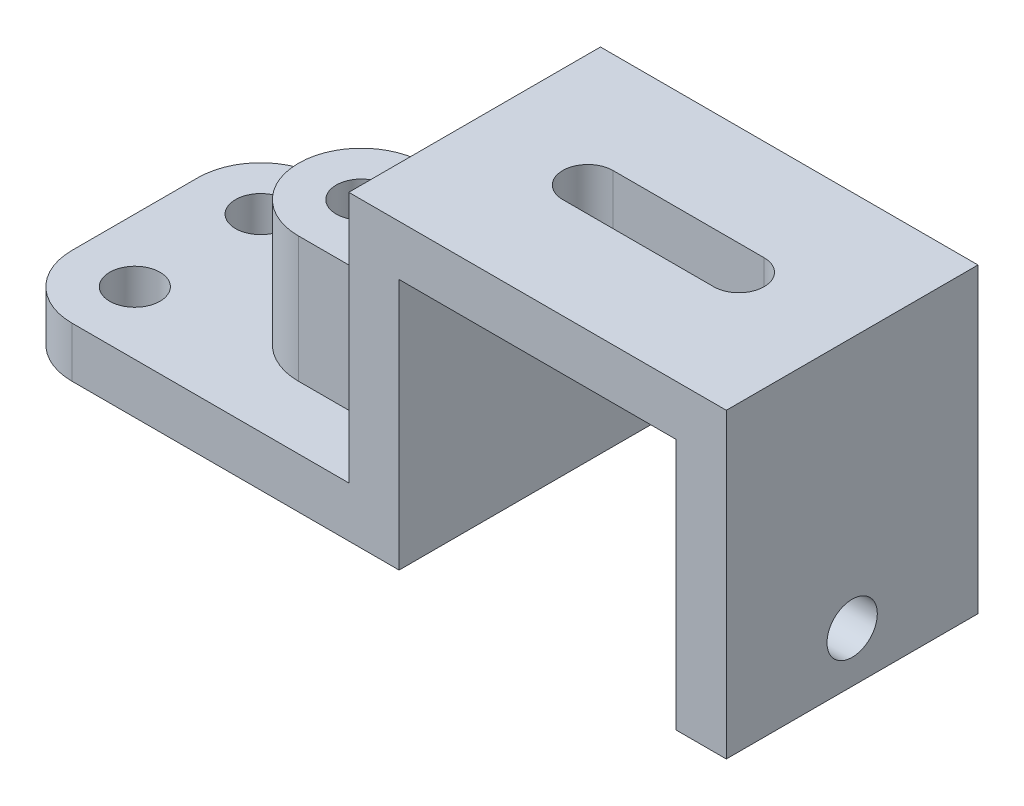
ISO-10303-21;
HEADER;
FILE_DESCRIPTION(('STEP AP214'),'2;1');
FILE_NAME('part.step','',(''),(''),'','','');
FILE_SCHEMA(('AUTOMOTIVE_DESIGN { 1 0 10303 214 1 1 1 1 }'));
ENDSEC;
DATA;
#1=APPLICATION_CONTEXT('core data for automotive mechanical design processes');
#2=APPLICATION_PROTOCOL_DEFINITION('international standard','automotive_design',2000,#1);
#3=PRODUCT_CONTEXT('',#1,'mechanical');
#4=PRODUCT('Part','Part','',(#3));
#5=PRODUCT_RELATED_PRODUCT_CATEGORY('part','',(#4));
#6=PRODUCT_DEFINITION_FORMATION('','',#4);
#7=PRODUCT_DEFINITION_CONTEXT('part definition',#1,'design');
#8=PRODUCT_DEFINITION('design','',#6,#7);
#9=PRODUCT_DEFINITION_SHAPE('','',#8);
#10=(LENGTH_UNIT() NAMED_UNIT(*) SI_UNIT(.MILLI.,.METRE.));
#11=(NAMED_UNIT(*) PLANE_ANGLE_UNIT() SI_UNIT($,.RADIAN.));
#12=(NAMED_UNIT(*) SI_UNIT($,.STERADIAN.) SOLID_ANGLE_UNIT());
#13=UNCERTAINTY_MEASURE_WITH_UNIT(LENGTH_MEASURE(1.E-05),#10,'distance_accuracy_value','');
#14=(GEOMETRIC_REPRESENTATION_CONTEXT(3) GLOBAL_UNCERTAINTY_ASSIGNED_CONTEXT((#13)) GLOBAL_UNIT_ASSIGNED_CONTEXT((#10,
#11,#12)) REPRESENTATION_CONTEXT('',''));
#15=CARTESIAN_POINT('',(0.,0.,0.));
#16=DIRECTION('',(0.,0.,1.));
#17=DIRECTION('',(1.,0.,0.));
#18=AXIS2_PLACEMENT_3D('',#15,#16,#17);
#19=CARTESIAN_POINT('',(121.5,17.9999999999999,45.));
#20=DIRECTION('',(1.,0.,0.));
#21=DIRECTION('',(0.,0.,-1.));
#22=AXIS2_PLACEMENT_3D('',#19,#20,#21);
#23=PLANE('',#22);
#24=DIRECTION('',(0.,-1.,0.));
#25=VECTOR('',#24,1.);
#26=CARTESIAN_POINT('',(121.5,62.9999999999999,22.5));
#27=LINE('',#26,#25);
#28=CARTESIAN_POINT('',(121.5,62.9999999999999,22.5));
#29=VERTEX_POINT('',#28);
#30=CARTESIAN_POINT('',(121.5,17.9999999999999,22.5));
#31=VERTEX_POINT('',#30);
#32=EDGE_CURVE('E187',#29,#31,#27,.T.);
#33=ORIENTED_EDGE('',*,*,#32,.T.);
#34=DIRECTION('',(0.,0.,-1.));
#35=VECTOR('',#34,1.);
#36=CARTESIAN_POINT('',(121.5,17.9999999999999,45.));
#37=LINE('',#36,#35);
#38=CARTESIAN_POINT('',(121.5,17.9999999999999,45.));
#39=VERTEX_POINT('',#38);
#40=EDGE_CURVE('E276',#39,#31,#37,.T.);
#41=ORIENTED_EDGE('',*,*,#40,.F.);
#42=DIRECTION('',(0.,-1.,0.));
#43=VECTOR('',#42,1.);
#44=CARTESIAN_POINT('',(121.5,17.9999999999999,45.));
#45=LINE('',#44,#43);
#46=CARTESIAN_POINT('',(121.5,108.,45.));
#47=VERTEX_POINT('',#46);
#48=EDGE_CURVE('E253',#47,#39,#45,.T.);
#49=ORIENTED_EDGE('',*,*,#48,.F.);
#50=DIRECTION('',(0.,0.,-1.));
#51=VECTOR('',#50,1.);
#52=CARTESIAN_POINT('',(121.5,108.,45.));
#53=LINE('',#52,#51);
#54=CARTESIAN_POINT('',(121.5,108.,-45.));
#55=VERTEX_POINT('',#54);
#56=EDGE_CURVE('E285',#47,#55,#53,.T.);
#57=ORIENTED_EDGE('',*,*,#56,.T.);
#58=DIRECTION('',(0.,-1.,0.));
#59=VECTOR('',#58,1.);
#60=CARTESIAN_POINT('',(121.5,17.9999999999999,-45.));
#61=LINE('',#60,#59);
#62=CARTESIAN_POINT('',(121.5,17.9999999999999,-45.));
#63=VERTEX_POINT('',#62);
#64=EDGE_CURVE('E267',#55,#63,#61,.T.);
#65=ORIENTED_EDGE('',*,*,#64,.T.);
#66=CARTESIAN_POINT('',(121.5,17.9999999999999,-22.4999999999999));
#67=VERTEX_POINT('',#66);
#68=EDGE_CURVE('E279',#67,#63,#37,.T.);
#69=ORIENTED_EDGE('',*,*,#68,.F.);
#70=DIRECTION('',(0.,-1.,0.));
#71=VECTOR('',#70,1.);
#72=CARTESIAN_POINT('',(121.5,62.9999999999999,-22.5));
#73=LINE('',#72,#71);
#74=CARTESIAN_POINT('',(121.5,62.9999999999999,-22.5));
#75=VERTEX_POINT('',#74);
#76=EDGE_CURVE('E211',#75,#67,#73,.T.);
#77=ORIENTED_EDGE('',*,*,#76,.F.);
#78=DIRECTION('',(0.,0.,-1.));
#79=VECTOR('',#78,1.);
#80=CARTESIAN_POINT('',(121.5,62.9999999999999,-22.5));
#81=LINE('',#80,#79);
#82=EDGE_CURVE('E191',#29,#75,#81,.T.);
#83=ORIENTED_EDGE('',*,*,#82,.F.);
#84=EDGE_LOOP('',(#33,#41,#49,#57,#65,#69,#77,#83));
#85=FACE_BOUND('',#84,.T.);
#86=ADVANCED_FACE('F39',(#85),#23,.F.);
#87=CARTESIAN_POINT('',(0.,17.9999999999999,45.));
#88=DIRECTION('',(0.,-1.,0.));
#89=DIRECTION('',(0.,0.,-1.));
#90=AXIS2_PLACEMENT_3D('',#87,#88,#89);
#91=PLANE('',#90);
#92=CARTESIAN_POINT('',(22.5,17.9999999999999,-22.5));
#93=DIRECTION('',(0.,1.,0.));
#94=DIRECTION('',(0.,0.,1.));
#95=AXIS2_PLACEMENT_3D('',#92,#93,#94);
#96=CIRCLE('',#95,9.);
#97=CARTESIAN_POINT('',(22.5,17.9999999999999,-13.5));
#98=VERTEX_POINT('',#97);
#99=EDGE_CURVE('E327',#98,#98,#96,.T.);
#100=ORIENTED_EDGE('',*,*,#99,.F.);
#101=EDGE_LOOP('',(#100));
#102=FACE_BOUND('',#101,.T.);
#103=CARTESIAN_POINT('',(22.5,17.9999999999999,22.5));
#104=DIRECTION('',(0.,1.,0.));
#105=DIRECTION('',(0.,0.,1.));
#106=AXIS2_PLACEMENT_3D('',#103,#104,#105);
#107=CIRCLE('',#106,9.);
#108=CARTESIAN_POINT('',(22.5,17.9999999999999,31.5));
#109=VERTEX_POINT('',#108);
#110=EDGE_CURVE('E331',#109,#109,#107,.T.);
#111=ORIENTED_EDGE('',*,*,#110,.F.);
#112=EDGE_LOOP('',(#111));
#113=FACE_BOUND('',#112,.T.);
#114=DIRECTION('',(-1.,0.,0.));
#115=VECTOR('',#114,1.);
#116=CARTESIAN_POINT('',(0.,17.9999999999999,-45.));
#117=LINE('',#116,#115);
#118=CARTESIAN_POINT('',(22.5,17.9999999999999,-45.));
#119=VERTEX_POINT('',#118);
#120=EDGE_CURVE('E239',#63,#119,#117,.T.);
#121=ORIENTED_EDGE('',*,*,#120,.T.);
#122=CARTESIAN_POINT('',(22.5,17.9999999999999,-22.5));
#123=DIRECTION('',(0.,-1.,0.));
#124=DIRECTION('',(0.,0.,-1.));
#125=AXIS2_PLACEMENT_3D('',#122,#123,#124);
#126=CIRCLE('',#125,22.5);
#127=CARTESIAN_POINT('',(0.,17.9999999999999,-22.5));
#128=VERTEX_POINT('',#127);
#129=EDGE_CURVE('E48',#119,#128,#126,.F.);
#130=ORIENTED_EDGE('',*,*,#129,.T.);
#131=DIRECTION('',(0.,0.,-1.));
#132=VECTOR('',#131,1.);
#133=CARTESIAN_POINT('',(0.,17.9999999999999,45.));
#134=LINE('',#133,#132);
#135=CARTESIAN_POINT('',(0.,17.9999999999999,22.5));
#136=VERTEX_POINT('',#135);
#137=EDGE_CURVE('E274',#136,#128,#134,.T.);
#138=ORIENTED_EDGE('',*,*,#137,.F.);
#139=CARTESIAN_POINT('',(22.5,17.9999999999999,22.5));
#140=DIRECTION('',(0.,-1.,0.));
#141=DIRECTION('',(0.,0.,-1.));
#142=AXIS2_PLACEMENT_3D('',#139,#140,#141);
#143=CIRCLE('',#142,22.5);
#144=CARTESIAN_POINT('',(22.5,17.9999999999999,45.));
#145=VERTEX_POINT('',#144);
#146=EDGE_CURVE('E57',#136,#145,#143,.F.);
#147=ORIENTED_EDGE('',*,*,#146,.T.);
#148=DIRECTION('',(-1.,0.,0.));
#149=VECTOR('',#148,1.);
#150=CARTESIAN_POINT('',(0.,17.9999999999999,45.));
#151=LINE('',#150,#149);
#152=EDGE_CURVE('E251',#39,#145,#151,.T.);
#153=ORIENTED_EDGE('',*,*,#152,.F.);
#154=ORIENTED_EDGE('',*,*,#40,.T.);
#155=DIRECTION('',(1.,0.,0.));
#156=VECTOR('',#155,1.);
#157=CARTESIAN_POINT('',(81.,17.9999999999999,22.5));
#158=LINE('',#157,#156);
#159=CARTESIAN_POINT('',(81.,17.9999999999999,22.5));
#160=VERTEX_POINT('',#159);
#161=EDGE_CURVE('E351',#160,#31,#158,.T.);
#162=ORIENTED_EDGE('',*,*,#161,.F.);
#163=CARTESIAN_POINT('',(81.,17.9999999999999,0.));
#164=DIRECTION('',(0.,1.,0.));
#165=DIRECTION('',(0.,0.,1.));
#166=AXIS2_PLACEMENT_3D('',#163,#164,#165);
#167=CIRCLE('',#166,22.5);
#168=CARTESIAN_POINT('',(81.,17.9999999999999,-22.5));
#169=VERTEX_POINT('',#168);
#170=EDGE_CURVE('E206',#169,#160,#167,.T.);
#171=ORIENTED_EDGE('',*,*,#170,.F.);
#172=DIRECTION('',(-1.,0.,0.));
#173=VECTOR('',#172,1.);
#174=CARTESIAN_POINT('',(81.,17.9999999999999,-22.5));
#175=LINE('',#174,#173);
#176=EDGE_CURVE('E201',#67,#169,#175,.T.);
#177=ORIENTED_EDGE('',*,*,#176,.F.);
#178=ORIENTED_EDGE('',*,*,#68,.T.);
#179=EDGE_LOOP('',(#121,#130,#138,#147,#153,#154,#162,#171,#177,#178));
#180=FACE_BOUND('',#179,.T.);
#181=ADVANCED_FACE('F361',(#102,#113,#180),#91,.F.);
#182=CARTESIAN_POINT('',(139.5,0.,45.));
#183=DIRECTION('',(0.,1.,0.));
#184=DIRECTION('',(-1.,0.,0.));
#185=AXIS2_PLACEMENT_3D('',#182,#183,#184);
#186=PLANE('',#185);
#187=CARTESIAN_POINT('',(22.5,0.,-22.5));
#188=DIRECTION('',(0.,1.,0.));
#189=DIRECTION('',(-1.,0.,0.));
#190=AXIS2_PLACEMENT_3D('',#187,#188,#189);
#191=CIRCLE('',#190,9.);
#192=CARTESIAN_POINT('',(13.5,0.,-22.5));
#193=VERTEX_POINT('',#192);
#194=EDGE_CURVE('E43',#193,#193,#191,.T.);
#195=ORIENTED_EDGE('',*,*,#194,.T.);
#196=EDGE_LOOP('',(#195));
#197=FACE_BOUND('',#196,.T.);
#198=CARTESIAN_POINT('',(22.5,0.,22.5));
#199=DIRECTION('',(0.,1.,0.));
#200=DIRECTION('',(-1.,0.,0.));
#201=AXIS2_PLACEMENT_3D('',#198,#199,#200);
#202=CIRCLE('',#201,9.);
#203=CARTESIAN_POINT('',(13.5,0.,22.5));
#204=VERTEX_POINT('',#203);
#205=EDGE_CURVE('E326',#204,#204,#202,.T.);
#206=ORIENTED_EDGE('',*,*,#205,.T.);
#207=EDGE_LOOP('',(#206));
#208=FACE_BOUND('',#207,.T.);
#209=CARTESIAN_POINT('',(81.,0.,0.));
#210=DIRECTION('',(0.,1.,0.));
#211=DIRECTION('',(-1.,0.,0.));
#212=AXIS2_PLACEMENT_3D('',#209,#210,#211);
#213=CIRCLE('',#212,9.);
#214=CARTESIAN_POINT('',(72.,0.,0.));
#215=VERTEX_POINT('',#214);
#216=EDGE_CURVE('E347',#215,#215,#213,.T.);
#217=ORIENTED_EDGE('',*,*,#216,.T.);
#218=EDGE_LOOP('',(#217));
#219=FACE_BOUND('',#218,.T.);
#220=DIRECTION('',(0.,0.,-1.));
#221=VECTOR('',#220,1.);
#222=CARTESIAN_POINT('',(0.,0.,45.));
#223=LINE('',#222,#221);
#224=CARTESIAN_POINT('',(0.,0.,22.5));
#225=VERTEX_POINT('',#224);
#226=CARTESIAN_POINT('',(0.,0.,-22.5));
#227=VERTEX_POINT('',#226);
#228=EDGE_CURVE('E254',#225,#227,#223,.T.);
#229=ORIENTED_EDGE('',*,*,#228,.T.);
#230=CARTESIAN_POINT('',(22.5,0.,-22.5));
#231=DIRECTION('',(0.,1.,0.));
#232=DIRECTION('',(-1.,0.,0.));
#233=AXIS2_PLACEMENT_3D('',#230,#231,#232);
#234=CIRCLE('',#233,22.5);
#235=CARTESIAN_POINT('',(22.5,0.,-45.));
#236=VERTEX_POINT('',#235);
#237=EDGE_CURVE('E325',#227,#236,#234,.F.);
#238=ORIENTED_EDGE('',*,*,#237,.T.);
#239=DIRECTION('',(1.,0.,0.));
#240=VECTOR('',#239,1.);
#241=CARTESIAN_POINT('',(139.5,0.,-45.));
#242=LINE('',#241,#240);
#243=CARTESIAN_POINT('',(139.5,0.,-45.));
#244=VERTEX_POINT('',#243);
#245=EDGE_CURVE('E232',#236,#244,#242,.T.);
#246=ORIENTED_EDGE('',*,*,#245,.T.);
#247=DIRECTION('',(0.,0.,-1.));
#248=VECTOR('',#247,1.);
#249=CARTESIAN_POINT('',(139.5,0.,45.));
#250=LINE('',#249,#248);
#251=CARTESIAN_POINT('',(139.5,0.,45.));
#252=VERTEX_POINT('',#251);
#253=EDGE_CURVE('E297',#252,#244,#250,.T.);
#254=ORIENTED_EDGE('',*,*,#253,.F.);
#255=DIRECTION('',(1.,0.,0.));
#256=VECTOR('',#255,1.);
#257=CARTESIAN_POINT('',(139.5,0.,45.));
#258=LINE('',#257,#256);
#259=CARTESIAN_POINT('',(22.5,0.,45.));
#260=VERTEX_POINT('',#259);
#261=EDGE_CURVE('E237',#260,#252,#258,.T.);
#262=ORIENTED_EDGE('',*,*,#261,.F.);
#263=CARTESIAN_POINT('',(22.5,0.,22.5));
#264=DIRECTION('',(0.,1.,0.));
#265=DIRECTION('',(-1.,0.,0.));
#266=AXIS2_PLACEMENT_3D('',#263,#264,#265);
#267=CIRCLE('',#266,22.5);
#268=EDGE_CURVE('E319',#260,#225,#267,.F.);
#269=ORIENTED_EDGE('',*,*,#268,.T.);
#270=EDGE_LOOP('',(#229,#238,#246,#254,#262,#269));
#271=FACE_BOUND('',#270,.T.);
#272=ADVANCED_FACE('F404',(#197,#208,#219,#271),#186,.F.);
#273=CARTESIAN_POINT('',(139.5,89.9999999999999,45.));
#274=DIRECTION('',(-1.,0.,0.));
#275=DIRECTION('',(0.,0.,1.));
#276=AXIS2_PLACEMENT_3D('',#273,#274,#275);
#277=PLANE('',#276);
#278=DIRECTION('',(0.,1.,0.));
#279=VECTOR('',#278,1.);
#280=CARTESIAN_POINT('',(139.5,89.9999999999999,-45.));
#281=LINE('',#280,#279);
#282=CARTESIAN_POINT('',(139.5,89.9999999999999,-45.));
#283=VERTEX_POINT('',#282);
#284=EDGE_CURVE('E260',#244,#283,#281,.T.);
#285=ORIENTED_EDGE('',*,*,#284,.T.);
#286=DIRECTION('',(0.,0.,-1.));
#287=VECTOR('',#286,1.);
#288=CARTESIAN_POINT('',(139.5,89.9999999999999,45.));
#289=LINE('',#288,#287);
#290=CARTESIAN_POINT('',(139.5,89.9999999999999,45.));
#291=VERTEX_POINT('',#290);
#292=EDGE_CURVE('E300',#291,#283,#289,.T.);
#293=ORIENTED_EDGE('',*,*,#292,.F.);
#294=DIRECTION('',(0.,1.,0.));
#295=VECTOR('',#294,1.);
#296=CARTESIAN_POINT('',(139.5,89.9999999999999,45.));
#297=LINE('',#296,#295);
#298=EDGE_CURVE('E236',#252,#291,#297,.T.);
#299=ORIENTED_EDGE('',*,*,#298,.F.);
#300=ORIENTED_EDGE('',*,*,#253,.T.);
#301=EDGE_LOOP('',(#285,#293,#299,#300));
#302=FACE_BOUND('',#301,.T.);
#303=ADVANCED_FACE('F397',(#302),#277,.F.);
#304=CARTESIAN_POINT('',(238.5,89.9999999999999,45.));
#305=DIRECTION('',(0.,1.,0.));
#306=DIRECTION('',(-1.,0.,0.));
#307=AXIS2_PLACEMENT_3D('',#304,#305,#306);
#308=PLANE('',#307);
#309=DIRECTION('',(-1.,0.,0.));
#310=VECTOR('',#309,1.);
#311=CARTESIAN_POINT('',(238.5,89.9999999999999,-9.00000000000001));
#312=LINE('',#311,#310);
#313=CARTESIAN_POINT('',(216.,89.9999999999999,-9.00000000000001));
#314=VERTEX_POINT('',#313);
#315=CARTESIAN_POINT('',(162.,89.9999999999999,-9.));
#316=VERTEX_POINT('',#315);
#317=EDGE_CURVE('E229',#314,#316,#312,.T.);
#318=ORIENTED_EDGE('',*,*,#317,.T.);
#319=CARTESIAN_POINT('',(162.,89.9999999999999,0.));
#320=DIRECTION('',(0.,1.,0.));
#321=DIRECTION('',(-1.,0.,0.));
#322=AXIS2_PLACEMENT_3D('',#319,#320,#321);
#323=CIRCLE('',#322,9.);
#324=CARTESIAN_POINT('',(162.,89.9999999999999,9.));
#325=VERTEX_POINT('',#324);
#326=EDGE_CURVE('E235',#316,#325,#323,.T.);
#327=ORIENTED_EDGE('',*,*,#326,.T.);
#328=DIRECTION('',(1.,0.,0.));
#329=VECTOR('',#328,1.);
#330=CARTESIAN_POINT('',(238.5,89.9999999999999,9.));
#331=LINE('',#330,#329);
#332=CARTESIAN_POINT('',(216.,89.9999999999999,9.00000000000001));
#333=VERTEX_POINT('',#332);
#334=EDGE_CURVE('E217',#325,#333,#331,.T.);
#335=ORIENTED_EDGE('',*,*,#334,.T.);
#336=CARTESIAN_POINT('',(216.,89.9999999999999,0.));
#337=DIRECTION('',(0.,1.,0.));
#338=DIRECTION('',(-1.,0.,0.));
#339=AXIS2_PLACEMENT_3D('',#336,#337,#338);
#340=CIRCLE('',#339,9.);
#341=EDGE_CURVE('E228',#333,#314,#340,.T.);
#342=ORIENTED_EDGE('',*,*,#341,.T.);
#343=EDGE_LOOP('',(#318,#327,#335,#342));
#344=FACE_BOUND('',#343,.T.);
#345=DIRECTION('',(1.,0.,0.));
#346=VECTOR('',#345,1.);
#347=CARTESIAN_POINT('',(238.5,89.9999999999999,-45.));
#348=LINE('',#347,#346);
#349=CARTESIAN_POINT('',(238.5,89.9999999999999,-45.));
#350=VERTEX_POINT('',#349);
#351=EDGE_CURVE('E259',#283,#350,#348,.T.);
#352=ORIENTED_EDGE('',*,*,#351,.T.);
#353=DIRECTION('',(0.,0.,-1.));
#354=VECTOR('',#353,1.);
#355=CARTESIAN_POINT('',(238.5,89.9999999999999,45.));
#356=LINE('',#355,#354);
#357=CARTESIAN_POINT('',(238.5,89.9999999999999,45.));
#358=VERTEX_POINT('',#357);
#359=EDGE_CURVE('E294',#358,#350,#356,.T.);
#360=ORIENTED_EDGE('',*,*,#359,.F.);
#361=DIRECTION('',(1.,0.,0.));
#362=VECTOR('',#361,1.);
#363=CARTESIAN_POINT('',(238.5,89.9999999999999,45.));
#364=LINE('',#363,#362);
#365=EDGE_CURVE('E243',#291,#358,#364,.T.);
#366=ORIENTED_EDGE('',*,*,#365,.F.);
#367=ORIENTED_EDGE('',*,*,#292,.T.);
#368=EDGE_LOOP('',(#352,#360,#366,#367));
#369=FACE_BOUND('',#368,.T.);
#370=ADVANCED_FACE('F392',(#344,#369),#308,.F.);
#371=CARTESIAN_POINT('',(238.5,0.,45.));
#372=DIRECTION('',(1.,0.,0.));
#373=DIRECTION('',(0.,0.,-1.));
#374=AXIS2_PLACEMENT_3D('',#371,#372,#373);
#375=PLANE('',#374);
#376=CARTESIAN_POINT('',(238.5,18.,0.));
#377=DIRECTION('',(1.,0.,0.));
#378=DIRECTION('',(0.,0.,-1.));
#379=AXIS2_PLACEMENT_3D('',#376,#377,#378);
#380=CIRCLE('',#379,9.);
#381=CARTESIAN_POINT('',(238.5,18.,-9.));
#382=VERTEX_POINT('',#381);
#383=EDGE_CURVE('E339',#382,#382,#380,.T.);
#384=ORIENTED_EDGE('',*,*,#383,.T.);
#385=EDGE_LOOP('',(#384));
#386=FACE_BOUND('',#385,.T.);
#387=DIRECTION('',(0.,-1.,0.));
#388=VECTOR('',#387,1.);
#389=CARTESIAN_POINT('',(238.5,0.,-45.));
#390=LINE('',#389,#388);
#391=CARTESIAN_POINT('',(238.5,0.,-45.));
#392=VERTEX_POINT('',#391);
#393=EDGE_CURVE('E261',#350,#392,#390,.T.);
#394=ORIENTED_EDGE('',*,*,#393,.T.);
#395=DIRECTION('',(0.,0.,-1.));
#396=VECTOR('',#395,1.);
#397=CARTESIAN_POINT('',(238.5,0.,45.));
#398=LINE('',#397,#396);
#399=CARTESIAN_POINT('',(238.5,0.,45.));
#400=VERTEX_POINT('',#399);
#401=EDGE_CURVE('E292',#400,#392,#398,.T.);
#402=ORIENTED_EDGE('',*,*,#401,.F.);
#403=DIRECTION('',(0.,-1.,0.));
#404=VECTOR('',#403,1.);
#405=CARTESIAN_POINT('',(238.5,0.,45.));
#406=LINE('',#405,#404);
#407=EDGE_CURVE('E241',#358,#400,#406,.T.);
#408=ORIENTED_EDGE('',*,*,#407,.F.);
#409=ORIENTED_EDGE('',*,*,#359,.T.);
#410=EDGE_LOOP('',(#394,#402,#408,#409));
#411=FACE_BOUND('',#410,.T.);
#412=ADVANCED_FACE('F388',(#386,#411),#375,.F.);
#413=CARTESIAN_POINT('',(256.5,0.,45.));
#414=DIRECTION('',(0.,1.,0.));
#415=DIRECTION('',(0.,0.,1.));
#416=AXIS2_PLACEMENT_3D('',#413,#414,#415);
#417=PLANE('',#416);
#418=DIRECTION('',(1.,0.,0.));
#419=VECTOR('',#418,1.);
#420=CARTESIAN_POINT('',(256.5,0.,-45.));
#421=LINE('',#420,#419);
#422=CARTESIAN_POINT('',(256.5,0.,-45.));
#423=VERTEX_POINT('',#422);
#424=EDGE_CURVE('E263',#392,#423,#421,.T.);
#425=ORIENTED_EDGE('',*,*,#424,.T.);
#426=DIRECTION('',(0.,0.,-1.));
#427=VECTOR('',#426,1.);
#428=CARTESIAN_POINT('',(256.5,0.,45.));
#429=LINE('',#428,#427);
#430=CARTESIAN_POINT('',(256.5,0.,45.));
#431=VERTEX_POINT('',#430);
#432=EDGE_CURVE('E286',#431,#423,#429,.T.);
#433=ORIENTED_EDGE('',*,*,#432,.F.);
#434=DIRECTION('',(1.,0.,0.));
#435=VECTOR('',#434,1.);
#436=CARTESIAN_POINT('',(256.5,0.,45.));
#437=LINE('',#436,#435);
#438=EDGE_CURVE('E242',#400,#431,#437,.T.);
#439=ORIENTED_EDGE('',*,*,#438,.F.);
#440=ORIENTED_EDGE('',*,*,#401,.T.);
#441=EDGE_LOOP('',(#425,#433,#439,#440));
#442=FACE_BOUND('',#441,.T.);
#443=ADVANCED_FACE('F387',(#442),#417,.F.);
#444=CARTESIAN_POINT('',(256.5,108.,45.));
#445=DIRECTION('',(-1.,0.,0.));
#446=DIRECTION('',(0.,0.,1.));
#447=AXIS2_PLACEMENT_3D('',#444,#445,#446);
#448=PLANE('',#447);
#449=CARTESIAN_POINT('',(256.5,18.,0.));
#450=DIRECTION('',(1.,0.,0.));
#451=DIRECTION('',(0.,0.,-1.));
#452=AXIS2_PLACEMENT_3D('',#449,#450,#451);
#453=CIRCLE('',#452,9.);
#454=CARTESIAN_POINT('',(256.5,18.,-9.));
#455=VERTEX_POINT('',#454);
#456=EDGE_CURVE('E648',#455,#455,#453,.T.);
#457=ORIENTED_EDGE('',*,*,#456,.F.);
#458=EDGE_LOOP('',(#457));
#459=FACE_BOUND('',#458,.T.);
#460=DIRECTION('',(0.,1.,0.));
#461=VECTOR('',#460,1.);
#462=CARTESIAN_POINT('',(256.5,108.,-45.));
#463=LINE('',#462,#461);
#464=CARTESIAN_POINT('',(256.5,108.,-45.));
#465=VERTEX_POINT('',#464);
#466=EDGE_CURVE('E264',#423,#465,#463,.T.);
#467=ORIENTED_EDGE('',*,*,#466,.T.);
#468=DIRECTION('',(0.,0.,-1.));
#469=VECTOR('',#468,1.);
#470=CARTESIAN_POINT('',(256.5,108.,45.));
#471=LINE('',#470,#469);
#472=CARTESIAN_POINT('',(256.5,108.,45.));
#473=VERTEX_POINT('',#472);
#474=EDGE_CURVE('E282',#473,#465,#471,.T.);
#475=ORIENTED_EDGE('',*,*,#474,.F.);
#476=DIRECTION('',(0.,1.,0.));
#477=VECTOR('',#476,1.);
#478=CARTESIAN_POINT('',(256.5,108.,45.));
#479=LINE('',#478,#477);
#480=EDGE_CURVE('E250',#431,#473,#479,.T.);
#481=ORIENTED_EDGE('',*,*,#480,.F.);
#482=ORIENTED_EDGE('',*,*,#432,.T.);
#483=EDGE_LOOP('',(#467,#475,#481,#482));
#484=FACE_BOUND('',#483,.T.);
#485=ADVANCED_FACE('F385',(#459,#484),#448,.F.);
#486=CARTESIAN_POINT('',(121.5,108.,45.));
#487=DIRECTION('',(0.,-1.,0.));
#488=DIRECTION('',(0.,0.,-1.));
#489=AXIS2_PLACEMENT_3D('',#486,#487,#488);
#490=PLANE('',#489);
#491=DIRECTION('',(-1.,0.,0.));
#492=VECTOR('',#491,1.);
#493=CARTESIAN_POINT('',(121.5,108.,9.00000000000001));
#494=LINE('',#493,#492);
#495=CARTESIAN_POINT('',(216.,108.,9.));
#496=VERTEX_POINT('',#495);
#497=CARTESIAN_POINT('',(162.,108.,9.00000000000001));
#498=VERTEX_POINT('',#497);
#499=EDGE_CURVE('E301',#496,#498,#494,.T.);
#500=ORIENTED_EDGE('',*,*,#499,.T.);
#501=CARTESIAN_POINT('',(162.,108.,0.));
#502=DIRECTION('',(0.,-1.,0.));
#503=DIRECTION('',(0.,0.,-1.));
#504=AXIS2_PLACEMENT_3D('',#501,#502,#503);
#505=CIRCLE('',#504,9.);
#506=CARTESIAN_POINT('',(162.,108.,-9.));
#507=VERTEX_POINT('',#506);
#508=EDGE_CURVE('E315',#498,#507,#505,.T.);
#509=ORIENTED_EDGE('',*,*,#508,.T.);
#510=DIRECTION('',(1.,0.,0.));
#511=VECTOR('',#510,1.);
#512=CARTESIAN_POINT('',(121.5,108.,-8.99999999999999));
#513=LINE('',#512,#511);
#514=CARTESIAN_POINT('',(216.,108.,-9.00000000000001));
#515=VERTEX_POINT('',#514);
#516=EDGE_CURVE('E310',#507,#515,#513,.T.);
#517=ORIENTED_EDGE('',*,*,#516,.T.);
#518=CARTESIAN_POINT('',(216.,108.,0.));
#519=DIRECTION('',(0.,-1.,0.));
#520=DIRECTION('',(0.,0.,-1.));
#521=AXIS2_PLACEMENT_3D('',#518,#519,#520);
#522=CIRCLE('',#521,9.);
#523=EDGE_CURVE('E308',#515,#496,#522,.T.);
#524=ORIENTED_EDGE('',*,*,#523,.T.);
#525=EDGE_LOOP('',(#500,#509,#517,#524));
#526=FACE_BOUND('',#525,.T.);
#527=DIRECTION('',(-1.,0.,0.));
#528=VECTOR('',#527,1.);
#529=CARTESIAN_POINT('',(121.5,108.,-45.));
#530=LINE('',#529,#528);
#531=EDGE_CURVE('E270',#465,#55,#530,.T.);
#532=ORIENTED_EDGE('',*,*,#531,.T.);
#533=ORIENTED_EDGE('',*,*,#56,.F.);
#534=DIRECTION('',(-1.,0.,0.));
#535=VECTOR('',#534,1.);
#536=CARTESIAN_POINT('',(121.5,108.,45.));
#537=LINE('',#536,#535);
#538=EDGE_CURVE('E249',#473,#47,#537,.T.);
#539=ORIENTED_EDGE('',*,*,#538,.F.);
#540=ORIENTED_EDGE('',*,*,#474,.T.);
#541=EDGE_LOOP('',(#532,#533,#539,#540));
#542=FACE_BOUND('',#541,.T.);
#543=ADVANCED_FACE('F374',(#526,#542),#490,.F.);
#544=CARTESIAN_POINT('',(0.,0.,45.));
#545=DIRECTION('',(1.,0.,0.));
#546=DIRECTION('',(0.,1.,0.));
#547=AXIS2_PLACEMENT_3D('',#544,#545,#546);
#548=PLANE('',#547);
#549=ORIENTED_EDGE('',*,*,#137,.T.);
#550=DIRECTION('',(0.,-1.,0.));
#551=VECTOR('',#550,1.);
#552=CARTESIAN_POINT('',(0.,0.,-22.5));
#553=LINE('',#552,#551);
#554=EDGE_CURVE('E320',#128,#227,#553,.T.);
#555=ORIENTED_EDGE('',*,*,#554,.T.);
#556=ORIENTED_EDGE('',*,*,#228,.F.);
#557=DIRECTION('',(0.,-1.,0.));
#558=VECTOR('',#557,1.);
#559=CARTESIAN_POINT('',(0.,0.,22.5));
#560=LINE('',#559,#558);
#561=EDGE_CURVE('E312',#225,#136,#560,.F.);
#562=ORIENTED_EDGE('',*,*,#561,.T.);
#563=EDGE_LOOP('',(#549,#555,#556,#562));
#564=FACE_BOUND('',#563,.T.);
#565=ADVANCED_FACE('F409',(#564),#548,.F.);
#566=CARTESIAN_POINT('',(0.,0.,45.));
#567=DIRECTION('',(0.,0.,-1.));
#568=DIRECTION('',(-1.,0.,0.));
#569=AXIS2_PLACEMENT_3D('',#566,#567,#568);
#570=PLANE('',#569);
#571=ORIENTED_EDGE('',*,*,#152,.T.);
#572=DIRECTION('',(0.,-1.,0.));
#573=VECTOR('',#572,1.);
#574=CARTESIAN_POINT('',(22.5,0.,45.));
#575=LINE('',#574,#573);
#576=EDGE_CURVE('E11',#145,#260,#575,.T.);
#577=ORIENTED_EDGE('',*,*,#576,.T.);
#578=ORIENTED_EDGE('',*,*,#261,.T.);
#579=ORIENTED_EDGE('',*,*,#298,.T.);
#580=ORIENTED_EDGE('',*,*,#365,.T.);
#581=ORIENTED_EDGE('',*,*,#407,.T.);
#582=ORIENTED_EDGE('',*,*,#438,.T.);
#583=ORIENTED_EDGE('',*,*,#480,.T.);
#584=ORIENTED_EDGE('',*,*,#538,.T.);
#585=ORIENTED_EDGE('',*,*,#48,.T.);
#586=EDGE_LOOP('',(#571,#577,#578,#579,#580,#581,#582,#583,#584,#585));
#587=FACE_BOUND('',#586,.T.);
#588=ADVANCED_FACE('F369',(#587),#570,.F.);
#589=CARTESIAN_POINT('',(0.,0.,-45.));
#590=DIRECTION('',(0.,0.,-1.));
#591=DIRECTION('',(-1.,0.,0.));
#592=AXIS2_PLACEMENT_3D('',#589,#590,#591);
#593=PLANE('',#592);
#594=ORIENTED_EDGE('',*,*,#245,.F.);
#595=DIRECTION('',(0.,-1.,0.));
#596=VECTOR('',#595,1.);
#597=CARTESIAN_POINT('',(22.5,17.9999999999999,-45.));
#598=LINE('',#597,#596);
#599=EDGE_CURVE('E64',#236,#119,#598,.F.);
#600=ORIENTED_EDGE('',*,*,#599,.T.);
#601=ORIENTED_EDGE('',*,*,#120,.F.);
#602=ORIENTED_EDGE('',*,*,#64,.F.);
#603=ORIENTED_EDGE('',*,*,#531,.F.);
#604=ORIENTED_EDGE('',*,*,#466,.F.);
#605=ORIENTED_EDGE('',*,*,#424,.F.);
#606=ORIENTED_EDGE('',*,*,#393,.F.);
#607=ORIENTED_EDGE('',*,*,#351,.F.);
#608=ORIENTED_EDGE('',*,*,#284,.F.);
#609=EDGE_LOOP('',(#594,#600,#601,#602,#603,#604,#605,#606,#607,#608));
#610=FACE_BOUND('',#609,.T.);
#611=ADVANCED_FACE('F378',(#610),#593,.T.);
#612=CARTESIAN_POINT('',(162.,62.9999999999999,0.));
#613=DIRECTION('',(0.,1.,0.));
#614=DIRECTION('',(0.,0.,1.));
#615=AXIS2_PLACEMENT_3D('',#612,#613,#614);
#616=CYLINDRICAL_SURFACE('',#615,9.);
#617=DIRECTION('',(0.,1.,0.));
#618=VECTOR('',#617,1.);
#619=CARTESIAN_POINT('',(162.,62.9999999999999,-9.));
#620=LINE('',#619,#618);
#621=EDGE_CURVE('E214',#316,#507,#620,.T.);
#622=ORIENTED_EDGE('',*,*,#621,.T.);
#623=ORIENTED_EDGE('',*,*,#508,.F.);
#624=DIRECTION('',(0.,1.,0.));
#625=VECTOR('',#624,1.);
#626=CARTESIAN_POINT('',(162.,62.9999999999999,9.));
#627=LINE('',#626,#625);
#628=EDGE_CURVE('E210',#325,#498,#627,.T.);
#629=ORIENTED_EDGE('',*,*,#628,.F.);
#630=ORIENTED_EDGE('',*,*,#326,.F.);
#631=EDGE_LOOP('',(#622,#623,#629,#630));
#632=FACE_BOUND('',#631,.T.);
#633=ADVANCED_FACE('F479',(#632),#616,.F.);
#634=CARTESIAN_POINT('',(162.,62.9999999999999,-9.));
#635=DIRECTION('',(0.,0.,-1.));
#636=DIRECTION('',(-1.,0.,0.));
#637=AXIS2_PLACEMENT_3D('',#634,#635,#636);
#638=PLANE('',#637);
#639=DIRECTION('',(0.,1.,0.));
#640=VECTOR('',#639,1.);
#641=CARTESIAN_POINT('',(216.,62.9999999999999,-9.00000000000001));
#642=LINE('',#641,#640);
#643=EDGE_CURVE('E218',#314,#515,#642,.T.);
#644=ORIENTED_EDGE('',*,*,#643,.T.);
#645=ORIENTED_EDGE('',*,*,#516,.F.);
#646=ORIENTED_EDGE('',*,*,#621,.F.);
#647=ORIENTED_EDGE('',*,*,#317,.F.);
#648=EDGE_LOOP('',(#644,#645,#646,#647));
#649=FACE_BOUND('',#648,.T.);
#650=ADVANCED_FACE('F474',(#649),#638,.F.);
#651=CARTESIAN_POINT('',(216.,62.9999999999999,0.));
#652=DIRECTION('',(0.,1.,0.));
#653=DIRECTION('',(0.,0.,1.));
#654=AXIS2_PLACEMENT_3D('',#651,#652,#653);
#655=CYLINDRICAL_SURFACE('',#654,9.);
#656=DIRECTION('',(0.,1.,0.));
#657=VECTOR('',#656,1.);
#658=CARTESIAN_POINT('',(216.,62.9999999999999,9.));
#659=LINE('',#658,#657);
#660=EDGE_CURVE('E207',#333,#496,#659,.T.);
#661=ORIENTED_EDGE('',*,*,#660,.T.);
#662=ORIENTED_EDGE('',*,*,#523,.F.);
#663=ORIENTED_EDGE('',*,*,#643,.F.);
#664=ORIENTED_EDGE('',*,*,#341,.F.);
#665=EDGE_LOOP('',(#661,#662,#663,#664));
#666=FACE_BOUND('',#665,.T.);
#667=ADVANCED_FACE('F476',(#666),#655,.F.);
#668=CARTESIAN_POINT('',(162.,62.9999999999999,9.));
#669=DIRECTION('',(0.,0.,1.));
#670=DIRECTION('',(1.,0.,0.));
#671=AXIS2_PLACEMENT_3D('',#668,#669,#670);
#672=PLANE('',#671);
#673=ORIENTED_EDGE('',*,*,#628,.T.);
#674=ORIENTED_EDGE('',*,*,#499,.F.);
#675=ORIENTED_EDGE('',*,*,#660,.F.);
#676=ORIENTED_EDGE('',*,*,#334,.F.);
#677=EDGE_LOOP('',(#673,#674,#675,#676));
#678=FACE_BOUND('',#677,.T.);
#679=ADVANCED_FACE('F475',(#678),#672,.F.);
#680=CARTESIAN_POINT('',(81.,62.9999999999999,0.));
#681=DIRECTION('',(0.,-1.,0.));
#682=DIRECTION('',(0.,0.,-1.));
#683=AXIS2_PLACEMENT_3D('',#680,#681,#682);
#684=CYLINDRICAL_SURFACE('',#683,22.5);
#685=ORIENTED_EDGE('',*,*,#170,.T.);
#686=DIRECTION('',(0.,-1.,0.));
#687=VECTOR('',#686,1.);
#688=CARTESIAN_POINT('',(81.,62.9999999999999,22.5));
#689=LINE('',#688,#687);
#690=CARTESIAN_POINT('',(81.,62.9999999999999,22.5));
#691=VERTEX_POINT('',#690);
#692=EDGE_CURVE('E186',#691,#160,#689,.T.);
#693=ORIENTED_EDGE('',*,*,#692,.F.);
#694=CARTESIAN_POINT('',(81.,62.9999999999999,0.));
#695=DIRECTION('',(0.,1.,0.));
#696=DIRECTION('',(0.,0.,1.));
#697=AXIS2_PLACEMENT_3D('',#694,#695,#696);
#698=CIRCLE('',#697,22.5);
#699=CARTESIAN_POINT('',(81.,62.9999999999999,-22.5));
#700=VERTEX_POINT('',#699);
#701=EDGE_CURVE('E194',#700,#691,#698,.T.);
#702=ORIENTED_EDGE('',*,*,#701,.F.);
#703=DIRECTION('',(0.,-1.,0.));
#704=VECTOR('',#703,1.);
#705=CARTESIAN_POINT('',(81.,62.9999999999999,-22.5));
#706=LINE('',#705,#704);
#707=EDGE_CURVE('E353',#700,#169,#706,.T.);
#708=ORIENTED_EDGE('',*,*,#707,.T.);
#709=EDGE_LOOP('',(#685,#693,#702,#708));
#710=FACE_BOUND('',#709,.T.);
#711=ADVANCED_FACE('F202',(#710),#684,.T.);
#712=CARTESIAN_POINT('',(81.,62.9999999999999,22.5));
#713=DIRECTION('',(0.,0.,-1.));
#714=DIRECTION('',(-1.,0.,0.));
#715=AXIS2_PLACEMENT_3D('',#712,#713,#714);
#716=PLANE('',#715);
#717=ORIENTED_EDGE('',*,*,#161,.T.);
#718=ORIENTED_EDGE('',*,*,#32,.F.);
#719=DIRECTION('',(1.,0.,0.));
#720=VECTOR('',#719,1.);
#721=CARTESIAN_POINT('',(81.,62.9999999999999,22.5));
#722=LINE('',#721,#720);
#723=EDGE_CURVE('E181',#691,#29,#722,.T.);
#724=ORIENTED_EDGE('',*,*,#723,.F.);
#725=ORIENTED_EDGE('',*,*,#692,.T.);
#726=EDGE_LOOP('',(#717,#718,#724,#725));
#727=FACE_BOUND('',#726,.T.);
#728=ADVANCED_FACE('F188',(#727),#716,.F.);
#729=CARTESIAN_POINT('',(81.,62.9999999999999,-22.5));
#730=DIRECTION('',(0.,0.,1.));
#731=DIRECTION('',(1.,0.,0.));
#732=AXIS2_PLACEMENT_3D('',#729,#730,#731);
#733=PLANE('',#732);
#734=ORIENTED_EDGE('',*,*,#176,.T.);
#735=ORIENTED_EDGE('',*,*,#707,.F.);
#736=DIRECTION('',(-1.,0.,0.));
#737=VECTOR('',#736,1.);
#738=CARTESIAN_POINT('',(81.,62.9999999999999,-22.5));
#739=LINE('',#738,#737);
#740=EDGE_CURVE('E200',#75,#700,#739,.T.);
#741=ORIENTED_EDGE('',*,*,#740,.F.);
#742=ORIENTED_EDGE('',*,*,#76,.T.);
#743=EDGE_LOOP('',(#734,#735,#741,#742));
#744=FACE_BOUND('',#743,.T.);
#745=ADVANCED_FACE('F359',(#744),#733,.F.);
#746=CARTESIAN_POINT('',(81.,62.9999999999999,0.));
#747=DIRECTION('',(0.,1.,0.));
#748=DIRECTION('',(0.,0.,1.));
#749=AXIS2_PLACEMENT_3D('',#746,#747,#748);
#750=PLANE('',#749);
#751=CARTESIAN_POINT('',(81.,62.9999999999999,0.));
#752=DIRECTION('',(0.,1.,0.));
#753=DIRECTION('',(0.,0.,1.));
#754=AXIS2_PLACEMENT_3D('',#751,#752,#753);
#755=CIRCLE('',#754,9.);
#756=CARTESIAN_POINT('',(81.,62.9999999999999,9.));
#757=VERTEX_POINT('',#756);
#758=EDGE_CURVE('E335',#757,#757,#755,.T.);
#759=ORIENTED_EDGE('',*,*,#758,.F.);
#760=EDGE_LOOP('',(#759));
#761=FACE_BOUND('',#760,.T.);
#762=ORIENTED_EDGE('',*,*,#701,.T.);
#763=ORIENTED_EDGE('',*,*,#723,.T.);
#764=ORIENTED_EDGE('',*,*,#82,.T.);
#765=ORIENTED_EDGE('',*,*,#740,.T.);
#766=EDGE_LOOP('',(#762,#763,#764,#765));
#767=FACE_BOUND('',#766,.T.);
#768=ADVANCED_FACE('F197',(#761,#767),#750,.T.);
#769=CARTESIAN_POINT('',(81.,-9.00000000000009,0.));
#770=DIRECTION('',(0.,1.,0.));
#771=DIRECTION('',(0.,0.,1.));
#772=AXIS2_PLACEMENT_3D('',#769,#770,#771);
#773=CYLINDRICAL_SURFACE('',#772,9.);
#774=ORIENTED_EDGE('',*,*,#758,.T.);
#775=EDGE_LOOP('',(#774));
#776=FACE_BOUND('',#775,.T.);
#777=ORIENTED_EDGE('',*,*,#216,.F.);
#778=EDGE_LOOP('',(#777));
#779=FACE_BOUND('',#778,.T.);
#780=ADVANCED_FACE('F421',(#776,#779),#773,.F.);
#781=CARTESIAN_POINT('',(22.5,0.,-22.5));
#782=DIRECTION('',(0.,1.,0.));
#783=DIRECTION('',(-1.,0.,0.));
#784=AXIS2_PLACEMENT_3D('',#781,#782,#783);
#785=CYLINDRICAL_SURFACE('',#784,22.5);
#786=ORIENTED_EDGE('',*,*,#129,.F.);
#787=ORIENTED_EDGE('',*,*,#599,.F.);
#788=ORIENTED_EDGE('',*,*,#237,.F.);
#789=ORIENTED_EDGE('',*,*,#554,.F.);
#790=EDGE_LOOP('',(#786,#787,#788,#789));
#791=FACE_BOUND('',#790,.T.);
#792=ADVANCED_FACE('F408',(#791),#785,.T.);
#793=CARTESIAN_POINT('',(22.5,0.,22.5));
#794=DIRECTION('',(0.,-1.,0.));
#795=DIRECTION('',(1.,0.,0.));
#796=AXIS2_PLACEMENT_3D('',#793,#794,#795);
#797=CYLINDRICAL_SURFACE('',#796,22.5);
#798=ORIENTED_EDGE('',*,*,#146,.F.);
#799=ORIENTED_EDGE('',*,*,#561,.F.);
#800=ORIENTED_EDGE('',*,*,#268,.F.);
#801=ORIENTED_EDGE('',*,*,#576,.F.);
#802=EDGE_LOOP('',(#798,#799,#800,#801));
#803=FACE_BOUND('',#802,.T.);
#804=ADVANCED_FACE('F41',(#803),#797,.T.);
#805=CARTESIAN_POINT('',(22.5,-54.0000000000001,22.5));
#806=DIRECTION('',(0.,1.,0.));
#807=DIRECTION('',(0.,0.,1.));
#808=AXIS2_PLACEMENT_3D('',#805,#806,#807);
#809=CYLINDRICAL_SURFACE('',#808,9.);
#810=ORIENTED_EDGE('',*,*,#110,.T.);
#811=EDGE_LOOP('',(#810));
#812=FACE_BOUND('',#811,.T.);
#813=ORIENTED_EDGE('',*,*,#205,.F.);
#814=EDGE_LOOP('',(#813));
#815=FACE_BOUND('',#814,.T.);
#816=ADVANCED_FACE('F414',(#812,#815),#809,.F.);
#817=CARTESIAN_POINT('',(22.5,-54.0000000000001,-22.5));
#818=DIRECTION('',(0.,1.,0.));
#819=DIRECTION('',(0.,0.,1.));
#820=AXIS2_PLACEMENT_3D('',#817,#818,#819);
#821=CYLINDRICAL_SURFACE('',#820,9.);
#822=ORIENTED_EDGE('',*,*,#99,.T.);
#823=EDGE_LOOP('',(#822));
#824=FACE_BOUND('',#823,.T.);
#825=ORIENTED_EDGE('',*,*,#194,.F.);
#826=EDGE_LOOP('',(#825));
#827=FACE_BOUND('',#826,.T.);
#828=ADVANCED_FACE('F419',(#824,#827),#821,.F.);
#829=CARTESIAN_POINT('',(184.5,18.,0.));
#830=DIRECTION('',(1.,0.,0.));
#831=DIRECTION('',(0.,0.,-1.));
#832=AXIS2_PLACEMENT_3D('',#829,#830,#831);
#833=CYLINDRICAL_SURFACE('',#832,9.);
#834=ORIENTED_EDGE('',*,*,#456,.T.);
#835=EDGE_LOOP('',(#834));
#836=FACE_BOUND('',#835,.T.);
#837=ORIENTED_EDGE('',*,*,#383,.F.);
#838=EDGE_LOOP('',(#837));
#839=FACE_BOUND('',#838,.T.);
#840=ADVANCED_FACE('F532',(#836,#839),#833,.F.);
#841=CLOSED_SHELL('',(#86,#181,#272,#303,#370,#412,#443,#485,#543,#565,#588,#611,#633,#650,#667,
#679,#711,#728,#745,#768,#780,#792,#804,#816,#828,#840));
#842=MANIFOLD_SOLID_BREP('B2',#841);
#843=ADVANCED_BREP_SHAPE_REPRESENTATION('',(#18,#842),#14);
#844=SHAPE_DEFINITION_REPRESENTATION(#9,#843);
ENDSEC;
END-ISO-10303-21;
